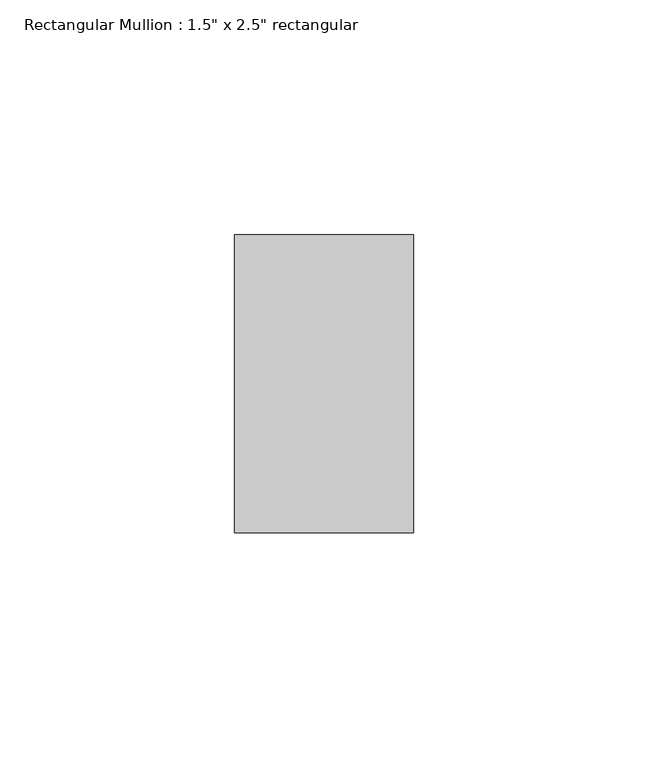
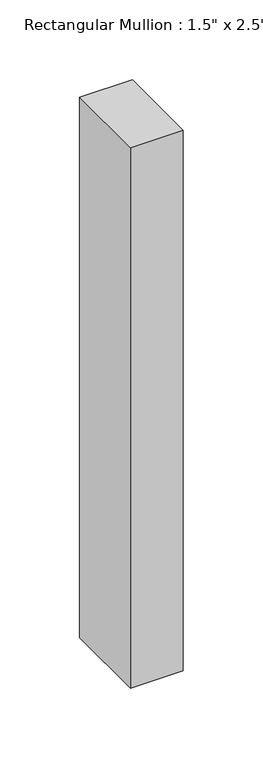
"""IFC4 building model written with IfcOpenShell, lengths in millimetres: member geometry."""

from ifc_helpers import new_model, si_unit, frame, origin, place, context, project, spatial, polyline, outline, extrude, source, transform, mapped, element, save


def member_5c5532da(model_context):
    return source(origin(), model_context, "Body", "SweptSolid", [
        extrude(outline(polyline([(0.0, 31.75), (0.0, -31.75), (-38.1, -31.75), (-38.1, 31.75), (0.0, 31.75)])), frame((0.0, 0.0, -413.2177198), z_axis=(0.0, 0.0, 1.0), x_axis=(1.0, 0.0, 0.0)), (0.0, 0.0, 1.0), 413.2177198),
    ])


if __name__ == "__main__":
    model = new_model("IFC4")
    model_context = context("Model", 3, world=origin())
    ifc_project = project(units=[si_unit("LENGTHUNIT", "METRE", prefix="MILLI")], contexts=[model_context])
    site = spatial("IfcSite", under=ifc_project)
    building = spatial("IfcBuilding", under=site)
    placement = place(None, origin())
    member_shape = member_5c5532da(model_context)
    element("IfcMember", 1, ObjectType="Rectangular Mullion : 1.5\" x 2.5\" rectangular", at=placement, inside=building, context=model_context, shape_type="MappedRepresentation", body=[
        mapped(member_shape, transform((0.0, 0.0, 0.0), x_axis=(1.0, 0.0, 0.0), y_axis=(0.0, 1.0, 0.0), z_axis=(0.0, 0.0, 1.0))),
    ])
    save(model, "model.ifc")

# Revit data of these elements
# Type "Rectangular Mullion : 1.5\" x 2.5\" rectangular"
#   built-in parameter 1007304 = 0.208333 (stored number, unit not read)
#   built-in parameter 1007301 = 0.0625 (stored number, unit not read)
#   built-in parameter 1007300 = 0.0625 (stored number, unit not read)
